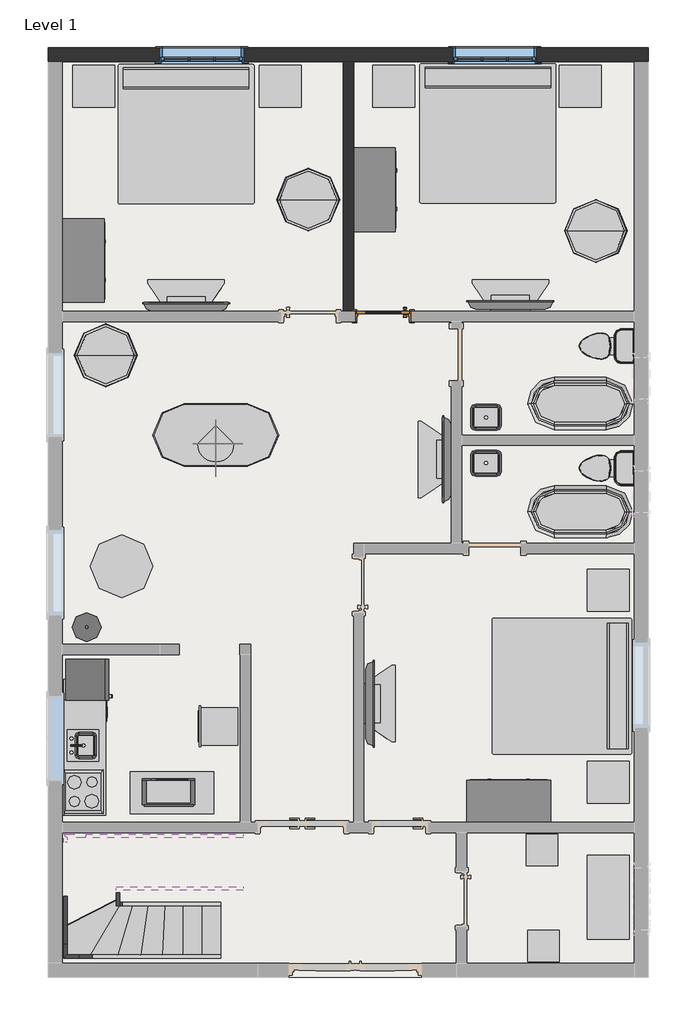
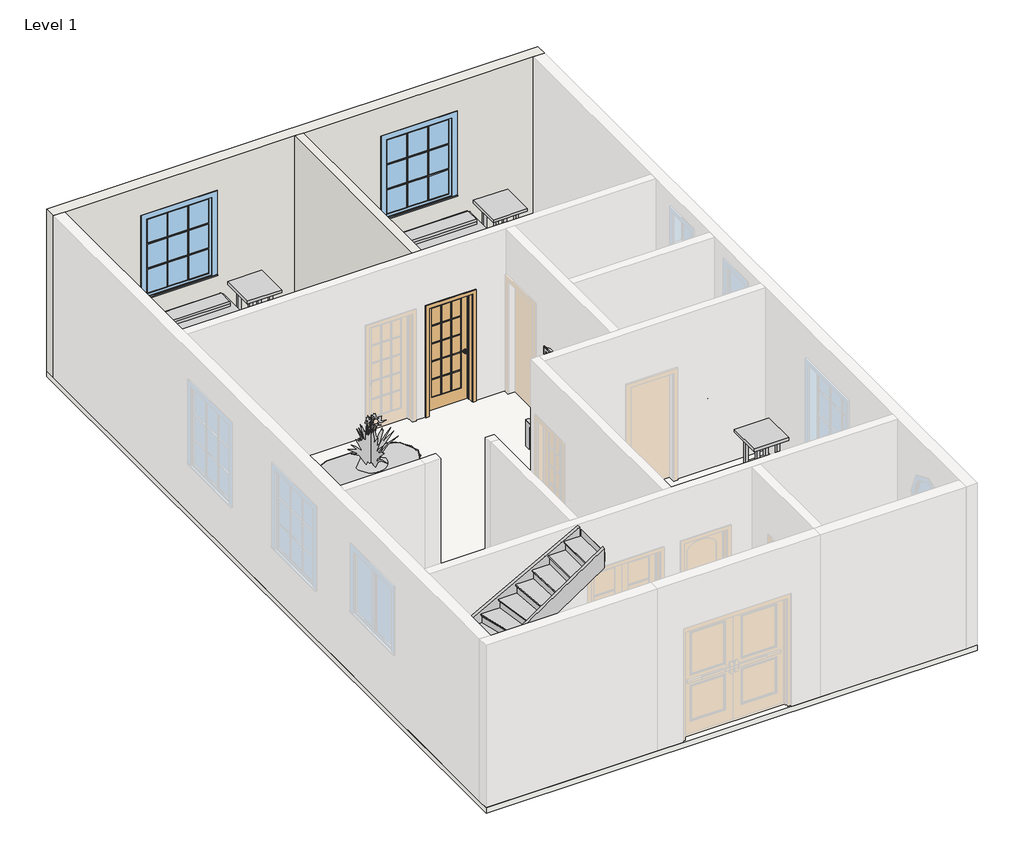
# One storey, part 2 of 2: 30 furniture elements, 10 members, 8 flow terminals, 6 proxies, 2 walls, 2 windows, 1 door, 1 geographic element, 2 other elements.
"""IFC4 building model written with IfcOpenShell, lengths in millimetres."""

from ifc_helpers import new_model, si_unit, frame, origin, origin_with_axes, place, context, project, spatial, polyline, outline, extrude, faceted_brep, transform, mapped, element, save
from components import proxy_a6faaae8, proxy_45b28599, kitchenette_medium_kitchenette_medium_844211aa, proxy_8a8d5ab2, proxy_34c9623a, proxy_c523a7b7, door_a0b5ff2a, flow_terminal_871c2e40, flow_terminal_d49f872f, flow_terminal_62a433f7, toilet_domestic_3d_toilet_domestic_3d_f7549cf7, toilet_domestic_3d_toilet_domestic_3d_183bbd19, flow_terminal_b374fae2, furniture_1fc5af50, furniture_1781b5df, furniture_9fa109b2, furniture_fdf74506, tv_stand_tv_stand_6ce107e5, furniture_2c34a4f9, furniture_905aceb5, furniture_097b63cf, furniture_5bc9ed15, furniture_51091a24, furniture_c80d6d9c, rpc_plant_tropical_55f6ff97, stair_flight_bf45dea3, window_cfa1ffdd

model = new_model("IFC4")

# Units and contexts
model_context = context("Model", 3, world=origin())
ifc_project = project(units=[si_unit("LENGTHUNIT", "METRE", prefix="MILLI")], contexts=[model_context])

# Site, building, storey
site = spatial("IfcSite", under=ifc_project)
building = spatial("IfcBuilding", under=site)
storey = spatial("IfcBuildingStorey", under=building, Name="Level 1", Elevation=0.0)

# Proxies
placement = place(None, origin())
proxy_shape = proxy_a6faaae8(model_context)
element("IfcBuildingElementProxy", 1, Name="Cook Top-4 Unit2 : 22\" x 20\"", ObjectType="Cook Top-4 Unit2 : 22\" x 20\"", at=placement, inside=storey, context=model_context, shape_type="MappedRepresentation", body=[
    mapped(proxy_shape, transform((-8710.4653968, 1396.1297533, 0.0), x_axis=(0.0, 1.0000000000000002, 0.0), y_axis=(-1.0000000000000002, 0.0, 0.0), z_axis=(0.0, 0.0, 1.0))),
])
proxy_2_shape = proxy_45b28599(model_context)
element("IfcBuildingElementProxy", 2, Name="Dishwasher : 24\" x 24\" x 34\"", ObjectType="Dishwasher : 24\" x 24\" x 34\"", at=placement, inside=storey, context=model_context, shape_type="MappedRepresentation", body=[
    mapped(proxy_2_shape, transform((-8418.6158321, 2347.3122848, 0.0), x_axis=(0.0, 1.0000000000000002, 0.0), y_axis=(-1.0000000000000002, 0.0, 0.0), z_axis=(0.0, 0.0, 1.0))),
])
kitchenette_medium_kitchenette_medium_shape = kitchenette_medium_kitchenette_medium_844211aa(model_context)
element("IfcBuildingElementProxy", 3, Name="Kitchenette - Medium : Kitchenette - Medium", ObjectType="Kitchenette - Medium : Kitchenette - Medium", at=placement, inside=storey, context=model_context, shape_type="MappedRepresentation", body=[
    mapped(kitchenette_medium_kitchenette_medium_shape, transform((-9015.2653968, 1720.2920484, 0.0), x_axis=(0.0, 1.0000000000000002, 0.0), y_axis=(-1.0000000000000002, 0.0, 0.0), z_axis=(0.0, 0.0, 1.0))),
])
proxy_3_shape = proxy_8a8d5ab2(model_context)
element("IfcBuildingElementProxy", 4, Name="Microwave : 30\" x 16\" x 18\"", ObjectType="Microwave : 30\" x 16\" x 18\"", at=placement, inside=storey, context=model_context, shape_type="MappedRepresentation", body=[
    mapped(proxy_3_shape, transform((-6965.5725195, 1030.3492475, 0.0), x_axis=(-1.0000000000000004, 0.0, 0.0), y_axis=(0.0, -1.0000000000000004, 0.0), z_axis=(0.0, 0.0, 1.0))),
])
proxy_4_shape = proxy_34c9623a(model_context)
element("IfcBuildingElementProxy", 5, Name="Oven Single-Built-in : 21\" x 23 1/2\" x 21\"", ObjectType="Oven Single-Built-in : 21\" x 23 1/2\" x 21\"", at=placement, inside=storey, context=model_context, shape_type="MappedRepresentation", body=[
    mapped(proxy_4_shape, transform((-6870.3312558, 2313.454826, 0.0), x_axis=(0.0, -1.0000000000000007, 0.0), y_axis=(1.0000000000000007, 0.0, 0.0), z_axis=(0.0, 0.0, 1.0))),
])
proxy_5_shape = proxy_c523a7b7(model_context)
element("IfcBuildingElementProxy", 6, Name="Refrigerator : 24\" x 25\" LH", ObjectType="Refrigerator : 24\" x 25\" LH", at=placement, inside=storey, context=model_context, shape_type="MappedRepresentation", body=[
    mapped(proxy_5_shape, transform((-8664.8164254, 3028.0797533, 0.0), x_axis=(0.0, 1.0000000000000002, 0.0), y_axis=(-1.0000000000000002, 0.0, 0.0), z_axis=(0.0, 0.0, 1.0))),
])

# Door
door_shape = door_a0b5ff2a(model_context)
element("IfcDoor", 7, ObjectType="Door-Interior-Single-Full Glass-Wood : 30\" x 80\"", at=placement, inside=storey, context=model_context, shape_type="MappedRepresentation", body=[
    mapped(door_shape, transform((-4341.6653968, 8320.8047533, 0.0), x_axis=(-1.0, 0.0, 0.0), y_axis=(0.0, -1.0, 0.0), z_axis=(0.0, 0.0, 1.0))),
])

# Flow terminals
flow_terminal_shape = flow_terminal_871c2e40(model_context)
element("IfcFlowTerminal", 8, ObjectType="Sink Kitchen-Island : 18\" x 18\"", at=placement, inside=storey, context=model_context, shape_type="MappedRepresentation", body=[
    mapped(flow_terminal_shape, transform((-8708.1199957, 2053.5405127, -14.4), x_axis=(0.0, 1.0000000000000002, 0.0), y_axis=(-1.0000000000000002, 0.0, 0.0), z_axis=(0.0, 0.0, 1.0))),
])
flow_terminal_2_shape = flow_terminal_d49f872f(model_context)
element("IfcFlowTerminal", 9, ObjectType="Sink Vanity-Round : 19\" x 19\"", at=placement, inside=storey, context=model_context, shape_type="MappedRepresentation", body=[
    mapped(flow_terminal_2_shape, transform((-8563.0136563, 3878.2665595, 609.6), x_axis=(-1.0000000000000004, 0.0, 0.0), y_axis=(0.0, -1.0000000000000004, 0.0), z_axis=(0.0, 0.0, 1.0))),
])
flow_terminal_3_shape = flow_terminal_62a433f7(model_context)
element("IfcFlowTerminal", 10, ObjectType="Sink Vanity-Square : 20\" x 18\"", at=placement, inside=storey, context=model_context, shape_type="MappedRepresentation", body=[
    mapped(flow_terminal_3_shape, transform((-2858.7546374, 6232.4843522, 609.6), x_axis=(1.0, 0.0, 0.0), y_axis=(0.0, 1.0, 0.0), z_axis=(0.0, 0.0, 1.0))),
])
element("IfcFlowTerminal", 11, ObjectType="Sink Vanity-Square : 20\" x 18\"", at=placement, inside=storey, context=model_context, shape_type="MappedRepresentation", body=[
    mapped(flow_terminal_3_shape, transform((-2827.3761563, 6795.9751544, 609.6), x_axis=(-1.0, 0.0, 0.0), y_axis=(0.0, -1.0, 0.0), z_axis=(0.0, 0.0, 1.0))),
])
toilet_domestic_3d_toilet_domestic_3d_shape = toilet_domestic_3d_toilet_domestic_3d_f7549cf7(model_context)
toilet_domestic_3d_toilet_domestic_3d_2_shape = toilet_domestic_3d_toilet_domestic_3d_183bbd19(model_context)
element("IfcFlowTerminal", 12, ObjectType="Toilet-Domestic-3D : Toilet-Domestic-3D", at=placement, inside=storey, context=model_context, shape_type="MappedRepresentation", body=[
    mapped(toilet_domestic_3d_toilet_domestic_3d_shape, transform((-1178.7614242, 7885.8297533, 0.0), x_axis=(0.0, -1.0000000000000002, 0.0), y_axis=(1.0000000000000002, 0.0, 0.0), z_axis=(0.0, 0.0, 1.0))),
    mapped(toilet_domestic_3d_toilet_domestic_3d_2_shape, transform((-1178.7614242, 7885.8297533, 0.0), x_axis=(0.0, -1.0000000000000002, 0.0), y_axis=(1.0000000000000002, 0.0, 0.0), z_axis=(0.0, 0.0, 1.0))),
])
element("IfcFlowTerminal", 13, ObjectType="Toilet-Domestic-3D : Toilet-Domestic-3D", at=placement, inside=storey, context=model_context, shape_type="MappedRepresentation", body=[
    mapped(toilet_domestic_3d_toilet_domestic_3d_shape, transform((-1178.7614242, 6107.8297533, 0.0), x_axis=(0.0, -1.0, 0.0), y_axis=(1.0, 0.0, 0.0), z_axis=(0.0, 0.0, 1.0))),
    mapped(toilet_domestic_3d_toilet_domestic_3d_2_shape, transform((-1178.7614242, 6107.8297533, 0.0), x_axis=(0.0, -1.0, 0.0), y_axis=(1.0, 0.0, 0.0), z_axis=(0.0, 0.0, 1.0))),
])
flow_terminal_4_shape = flow_terminal_b374fae2(model_context)
element("IfcFlowTerminal", 14, ObjectType="Tub-Free Standing-3D : 30\" x 60\"", at=placement, inside=storey, context=model_context, shape_type="MappedRepresentation", body=[
    mapped(flow_terminal_4_shape, transform((-1471.4653968, 7047.6297533, 0.0), x_axis=(0.0, -1.0000000000000002, 0.0), y_axis=(1.0000000000000002, 0.0, 0.0), z_axis=(0.0, 0.0, 1.0))),
])
element("IfcFlowTerminal", 15, ObjectType="Tub-Free Standing-3D : 30\" x 60\"", at=placement, inside=storey, context=model_context, shape_type="MappedRepresentation", body=[
    mapped(flow_terminal_4_shape, transform((-1471.4653968, 5472.8297533, 0.0), x_axis=(0.0, -1.0, 0.0), y_axis=(1.0, 0.0, 0.0), z_axis=(0.0, 0.0, 1.0))),
])

# Furniture
furniture_shape = furniture_1fc5af50(model_context)
element("IfcFurniture", 16, ObjectType="Bed-Standard.0001 : King 78\" x 80\"", at=placement, inside=storey, context=model_context, shape_type="MappedRepresentation", body=[
    mapped(furniture_shape, transform((-7483.3539214, 11017.5248353, 0.0), x_axis=(1.0, 0.0, 0.0), y_axis=(0.0, 1.0, 0.0), z_axis=(0.0, 0.0, 1.0))),
])
element("IfcFurniture", 17, ObjectType="Bed-Standard.0001 : King 78\" x 80\"", at=placement, inside=storey, context=model_context, shape_type="MappedRepresentation", body=[
    mapped(furniture_shape, transform((-3089.1539214, 11030.2248353, 0.0), x_axis=(1.0, 0.0, 0.0), y_axis=(0.0, 1.0, 0.0), z_axis=(0.0, 0.0, 1.0))),
])
element("IfcFurniture", 18, ObjectType="Bed-Standard.0001 : King 78\" x 80\"", at=placement, inside=storey, context=model_context, shape_type="MappedRepresentation", body=[
    mapped(furniture_shape, transform((-1692.5703149, 3204.3182779, 0.0), x_axis=(0.0, -1.0000000000000004, 0.0), y_axis=(1.0000000000000004, 0.0, 0.0), z_axis=(0.0, 0.0, 1.0))),
])
furniture_2_shape = furniture_1781b5df(model_context)
element("IfcFurniture", 19, ObjectType="Counter Top w Sink Hole : 24\" Depth", at=placement, inside=storey, context=model_context, shape_type="MappedRepresentation", body=[
    mapped(furniture_2_shape, transform((-9015.2653968, 2253.6920484, -14.4), x_axis=(0.0, 1.0000000000000002, 0.0), y_axis=(-1.0000000000000002, 0.0, 0.0), z_axis=(0.0, 0.0, 1.0))),
])
furniture_3_shape = furniture_9fa109b2(model_context)
element("IfcFurniture", 20, ObjectType="Dresser : 48\" x 72\" x 24\"", at=placement, inside=storey, context=model_context, shape_type="MappedRepresentation", body=[
    mapped(furniture_3_shape, transform((-9073.6283509, 9399.6230131, 0.0), x_axis=(0.0, 1.0000000000000002, 0.0), y_axis=(-1.0000000000000002, 0.0, 0.0), z_axis=(0.0, 0.0, 1.0))),
])
element("IfcFurniture", 21, ObjectType="Dresser : 48\" x 72\" x 24\"", at=placement, inside=storey, context=model_context, shape_type="MappedRepresentation", body=[
    mapped(furniture_3_shape, transform((-4831.8283509, 10430.8404811, 0.0), x_axis=(0.0, 1.0000000000000002, 0.0), y_axis=(-1.0000000000000002, 0.0, 0.0), z_axis=(0.0, 0.0, 1.0))),
])
element("IfcFurniture", 22, ObjectType="Dresser : 48\" x 72\" x 24\"", at=placement, inside=storey, context=model_context, shape_type="MappedRepresentation", body=[
    mapped(furniture_3_shape, transform((-2782.0586567, 893.2667992, 0.0), x_axis=(-1.0000000000000002, 0.0, 0.0), y_axis=(0.0, -1.0000000000000002, 0.0), z_axis=(0.0, 0.0, 1.0))),
])
furniture_4_shape = furniture_fdf74506(model_context)
element("IfcFurniture", 23, ObjectType="TV - Flat Screen : 50\"", at=placement, inside=storey, context=model_context, shape_type="MappedRepresentation", body=[
    mapped(furniture_4_shape, transform((-7215.809911, 8452.3683769, 914.4), x_axis=(-1.0, 0.0, 0.0), y_axis=(0.0, -1.0, 0.0), z_axis=(0.0, 0.0, 1.0))),
])
element("IfcFurniture", 24, ObjectType="TV - Flat Screen : 50\"", at=placement, inside=storey, context=model_context, shape_type="MappedRepresentation", body=[
    mapped(furniture_4_shape, transform((-2491.409911, 8477.7683769, 914.4), x_axis=(-1.0, 0.0, 0.0), y_axis=(0.0, -1.0, 0.0), z_axis=(0.0, 0.0, 1.0))),
])
element("IfcFurniture", 25, ObjectType="TV - Flat Screen : 50\"", at=placement, inside=storey, context=model_context, shape_type="MappedRepresentation", body=[
    mapped(furniture_4_shape, transform((-4537.1267732, 2682.7742674, 914.4), x_axis=(0.0, 1.0000000000000002, 0.0), y_axis=(-1.0000000000000002, 0.0, 0.0), z_axis=(0.0, 0.0, 1.0))),
])
element("IfcFurniture", 26, ObjectType="TV - Flat Screen : 50\"", at=placement, inside=storey, context=model_context, shape_type="MappedRepresentation", body=[
    mapped(furniture_4_shape, transform((-3409.6040205, 6230.8852392, 914.4), x_axis=(0.0, -1.0000000000000002, 0.0), y_axis=(1.0000000000000002, 0.0, 0.0), z_axis=(0.0, 0.0, 1.0))),
])
tv_stand_tv_stand_shape = tv_stand_tv_stand_6ce107e5(model_context)
element("IfcFurniture", 27, ObjectType="TV Stand : TV Stand", at=placement, inside=storey, context=model_context, shape_type="MappedRepresentation", body=[
    mapped(tv_stand_tv_stand_shape, transform((-7086.6773948, 8393.8297533, 0.0), x_axis=(-1.0000000000000004, 0.0, 0.0), y_axis=(0.0, -1.0000000000000004, 0.0), z_axis=(0.0, 0.0, 1.0))),
])
element("IfcFurniture", 28, ObjectType="TV Stand : TV Stand", at=placement, inside=storey, context=model_context, shape_type="MappedRepresentation", body=[
    mapped(tv_stand_tv_stand_shape, transform((-2362.2773948, 8393.8297533, 0.0), x_axis=(-1.0, 0.0, 0.0), y_axis=(0.0, -1.0, 0.0), z_axis=(0.0, 0.0, 1.0))),
])
element("IfcFurniture", 29, ObjectType="TV Stand : TV Stand", at=placement, inside=storey, context=model_context, shape_type="MappedRepresentation", body=[
    mapped(tv_stand_tv_stand_shape, transform((-4621.0653968, 2553.6417512, 0.0), x_axis=(0.0, 1.0000000000000004, 0.0), y_axis=(-1.0000000000000004, 0.0, 0.0), z_axis=(0.0, 0.0, 1.0))),
])
element("IfcFurniture", 30, ObjectType="TV Stand : TV Stand", at=placement, inside=storey, context=model_context, shape_type="MappedRepresentation", body=[
    mapped(tv_stand_tv_stand_shape, transform((-3376.4653968, 6360.0177554, 0.0), x_axis=(0.0, -1.0, 0.0), y_axis=(1.0, 0.0, 0.0), z_axis=(0.0, 0.0, 1.0))),
])
furniture_5_shape = furniture_2c34a4f9(model_context)
element("IfcFurniture", 31, ObjectType="Table-Dining Oval : 36\" x 72\"", at=placement, inside=storey, context=model_context, shape_type="MappedRepresentation", body=[
    mapped(furniture_5_shape, transform((-6378.2457247, 6948.528114, 0.0), x_axis=(1.0, 0.0, 0.0), y_axis=(0.0, 1.0, 0.0), z_axis=(0.0, 0.0, 1.0))),
])
furniture_6_shape = furniture_905aceb5(model_context)
element("IfcFurniture", 32, ObjectType="Table-Dining Round w Chairs : 36\" Diameter", at=placement, inside=storey, context=model_context, shape_type="MappedRepresentation", body=[
    mapped(furniture_6_shape, transform((-8255.3473641, 4863.9584418, 0.0), x_axis=(1.0, 0.0, 0.0), y_axis=(0.0, 1.0, 0.0), z_axis=(0.0, 0.0, 1.0))),
])
furniture_7_shape = furniture_097b63cf(model_context)
element("IfcFurniture", 33, ObjectType="Table-Night Stand : 18\" x 18\" x 24\"", at=placement, inside=storey, context=model_context, shape_type="MappedRepresentation", body=[
    mapped(furniture_7_shape, transform((-2262.5990271, 316.6297533, 0.0), x_axis=(1.0, 0.0, 0.0), y_axis=(0.0, 1.0, 0.0), z_axis=(0.0, 0.0, 1.0))),
])
element("IfcFurniture", 34, ObjectType="Table-Night Stand : 18\" x 18\" x 24\"", at=placement, inside=storey, context=model_context, shape_type="MappedRepresentation", body=[
    mapped(furniture_7_shape, transform((-2237.1990271, -1080.3702467, 0.0), x_axis=(1.0, 0.0, 0.0), y_axis=(0.0, 1.0, 0.0), z_axis=(0.0, 0.0, 1.0))),
])
furniture_8_shape = furniture_5bc9ed15(model_context)
element("IfcFurniture", 35, ObjectType="Table-Night Stand : 24\" x 24\" x 30\"", at=placement, inside=storey, context=model_context, shape_type="MappedRepresentation", body=[
    mapped(furniture_8_shape, transform((-1373.5990271, 4025.0297533, 0.0), x_axis=(1.0, 0.0, 0.0), y_axis=(0.0, 1.0, 0.0), z_axis=(0.0, 0.0, 1.0))),
])
element("IfcFurniture", 36, ObjectType="Table-Night Stand : 24\" x 24\" x 30\"", at=placement, inside=storey, context=model_context, shape_type="MappedRepresentation", body=[
    mapped(furniture_8_shape, transform((-1373.5990271, 1231.0297533, 0.0), x_axis=(1.0, 0.0, 0.0), y_axis=(0.0, 1.0, 0.0), z_axis=(0.0, 0.0, 1.0))),
])
element("IfcFurniture", 37, ObjectType="Table-Night Stand : 24\" x 24\" x 30\"", at=placement, inside=storey, context=model_context, shape_type="MappedRepresentation", body=[
    mapped(furniture_8_shape, transform((-8866.5990271, 11365.6297533, 0.0), x_axis=(1.0, 0.0, 0.0), y_axis=(0.0, 1.0, 0.0), z_axis=(0.0, 0.0, 1.0))),
])
element("IfcFurniture", 38, ObjectType="Table-Night Stand : 24\" x 24\" x 30\"", at=placement, inside=storey, context=model_context, shape_type="MappedRepresentation", body=[
    mapped(furniture_8_shape, transform((-6148.7990271, 11365.6297533, 0.0), x_axis=(1.0, 0.0, 0.0), y_axis=(0.0, 1.0, 0.0), z_axis=(0.0, 0.0, 1.0))),
])
element("IfcFurniture", 39, ObjectType="Table-Night Stand : 24\" x 24\" x 30\"", at=placement, inside=storey, context=model_context, shape_type="MappedRepresentation", body=[
    mapped(furniture_8_shape, transform((-4497.7990271, 11365.6297533, 0.0), x_axis=(1.0, 0.0, 0.0), y_axis=(0.0, 1.0, 0.0), z_axis=(0.0, 0.0, 1.0))),
])
element("IfcFurniture", 40, ObjectType="Table-Night Stand : 24\" x 24\" x 30\"", at=placement, inside=storey, context=model_context, shape_type="MappedRepresentation", body=[
    mapped(furniture_8_shape, transform((-1779.9990271, 11365.6297533, 0.0), x_axis=(1.0, 0.0, 0.0), y_axis=(0.0, 1.0, 0.0), z_axis=(0.0, 0.0, 1.0))),
])
furniture_9_shape = furniture_51091a24(model_context)
element("IfcFurniture", 41, ObjectType="Table-Rectangular : 72\" x 30\"", at=placement, inside=storey, context=model_context, shape_type="MappedRepresentation", body=[
    mapped(furniture_9_shape, transform((-1065.0653968, -140.5702467, 0.0), x_axis=(0.0, 1.0000000000000002, 0.0), y_axis=(-1.0000000000000002, 0.0, 0.0), z_axis=(0.0, 0.0, 1.0))),
])
element("IfcFurniture", 42, ObjectType="Table-Rectangular : 72\" x 30\"", at=placement, inside=storey, context=model_context, shape_type="MappedRepresentation", body=[
    mapped(furniture_9_shape, transform((-7415.0653968, 1383.4297533, 0.0), x_axis=(1.0, 0.0, 0.0), y_axis=(0.0, 1.0, 0.0), z_axis=(0.0, 0.0, 1.0))),
])
furniture_10_shape = furniture_c80d6d9c(model_context)
element("IfcFurniture", 43, ObjectType="Table-Round : 36\" Diameter", at=placement, inside=storey, context=model_context, shape_type="MappedRepresentation", body=[
    mapped(furniture_10_shape, transform((-5433.8653968, 10019.4297533, 0.0), x_axis=(1.0, 0.0, 0.0), y_axis=(0.0, 1.0, 0.0), z_axis=(0.0, 0.0, 1.0))),
])
element("IfcFurniture", 44, ObjectType="Table-Round : 36\" Diameter", at=placement, inside=storey, context=model_context, shape_type="MappedRepresentation", body=[
    mapped(furniture_10_shape, transform((-1242.8653968, 9562.2297533, 0.0), x_axis=(1.0, 0.0, 0.0), y_axis=(0.0, 1.0, 0.0), z_axis=(0.0, 0.0, 1.0))),
])
element("IfcFurniture", 45, ObjectType="Table-Round : 36\" Diameter", at=placement, inside=storey, context=model_context, shape_type="MappedRepresentation", body=[
    mapped(furniture_10_shape, transform((-8380.2653968, 7752.4797533, 0.0), x_axis=(1.0, 0.0, 0.0), y_axis=(0.0, 1.0, 0.0), z_axis=(0.0, 0.0, 1.0))),
])

# Geographic element
rpc_plant_tropical_shape = rpc_plant_tropical_55f6ff97(model_context)
element("IfcGeographicElement", 46, ObjectType="RPC Plant - Tropical", at=placement, inside=storey, context=model_context, shape_type="MappedRepresentation", body=[
    mapped(rpc_plant_tropical_shape, transform((-6780.0653968, 6463.4297533, 914.4), x_axis=(1.0, 0.0, 0.0), y_axis=(0.0, 1.0, 0.0), z_axis=(0.0, 0.0, 1.0))),
])

# Members
element("IfcMember", 47, ObjectType="Stringer - 2\" Width", at=placement, inside=storey, context=model_context, shape_type="SweptSolid", body=[
    extrude(outline(polyline([(0.0, -6703.8653968), (228.5330317, -6703.8653968), (1305.4011192, -8771.2543536), (961.730602, -8771.2543536), (0.0, -6924.9082236), (0.0, -6703.8653968)])), frame((0.0, -1029.5702467, 0.0), z_axis=(0.0, 1.0, 0.0), x_axis=(0.0, 0.0, 1.0)), (0.0, 0.0, 1.0), 50.8),
])
element("IfcMember", 48, ObjectType="Stringer - 2\" Width", at=placement, inside=storey, context=model_context, shape_type="SweptSolid", body=[
    extrude(outline(polyline([(-8771.2543536, -978.7702467), (-8771.2543536, -1029.5702467), (-8993.5970887, -1029.5702467), (-8942.7970887, -978.7702467), (-8771.2543536, -978.7702467)])), frame((0.0, 0.0, 961.730602), z_axis=(0.0, 0.0, 1.0), x_axis=(1.0, 0.0, 0.0)), (0.0, 0.0, 1.0), 343.6705172),
])
element("IfcMember", 49, ObjectType="Stringer - 2\" Width", at=placement, inside=storey, context=model_context, shape_type="SweptSolid", body=[
    extrude(outline(polyline([(-8942.7970887, -978.7702467), (-8993.5970887, -1029.5702467), (-8993.5970887, -827.9218653), (-8942.7970887, -827.9218653), (-8942.7970887, -978.7702467)])), frame((0.0, 0.0, 961.730602), z_axis=(0.0, 0.0, 1.0), x_axis=(1.0, 0.0, 0.0)), (0.0, 0.0, 1.0), 343.6705172),
])
element("IfcMember", 50, ObjectType="Stringer - 2\" Width", at=placement, inside=storey, context=model_context, shape_type="SweptSolid", body=[
    extrude(outline(polyline([(-827.9218653, 961.730602), (-827.9218653, 1305.4011192), (662.2844822, 1813.4011192), (662.2844822, 1469.730602), (-827.9218653, 961.730602)])), frame((-8993.5970887, 0.0, 0.0), z_axis=(1.0, 0.0, 0.0), x_axis=(0.0, 1.0, 0.0)), (0.0, 0.0, 1.0), 50.8),
])
element("IfcMember", 51, ObjectType="Stringer - 2\" Width", at=placement, inside=storey, context=model_context, shape_type="SweptSolid", body=[
    extrude(outline(polyline([(-8942.7970887, 662.2844822), (-8993.5970887, 662.2844822), (-8993.5970887, 773.8297533), (-8942.7970887, 723.0297533), (-8942.7970887, 662.2844822)])), frame((0.0, 0.0, 1479.9551215), z_axis=(0.0, 0.0, 1.0), x_axis=(1.0, 0.0, 0.0)), (0.0, 0.0, 1.0), 322.0234171),
])
element("IfcMember", 52, ObjectType="Stringer - 2\" Width", at=placement, inside=storey, context=model_context, shape_type="SweptSolid", body=[
    extrude(outline(polyline([(0.0, -6703.8653968), (194.5849337, -6703.8653968), (1234.3238531, -8180.7970887), (861.5700283, -8180.7970887), (0.0, -6956.9513176), (0.0, -6703.8653968)])), frame((0.0, -267.5702467, 0.0), z_axis=(0.0, 1.0, 0.0), x_axis=(0.0, 0.0, 1.0)), (0.0, 0.0, 1.0), 50.8),
])
element("IfcMember", 53, ObjectType="Stringer - 2\" Width", at=placement, inside=storey, context=model_context, shape_type="SweptSolid", body=[
    extrude(outline(polyline([(-267.5702467, 897.3325063), (-267.5702467, 1478.2726464), (-53.2751767, 1871.3232191), (-38.9702467, 1871.3232191), (-38.9702467, 1260.8183928), (-237.1463566, 897.3325063), (-267.5702467, 897.3325063)])), frame((-8231.5970887, 0.0, 0.0), z_axis=(1.0, 0.0, 0.0), x_axis=(0.0, 1.0, 0.0)), (0.0, 0.0, 1.0), 50.8),
])
element("IfcMember", 54, ObjectType="Stringer - 2\" Width", at=placement, inside=storey, context=model_context, shape_type="SweptSolid", body=[
    extrude(outline(polyline([(1871.3232191, -8231.5970887), (1503.9377762, -8231.5970887), (2748.6444185, -6381.8994015), (3116.0298613, -6381.8994015), (1871.3232191, -8231.5970887)])), frame((0.0, -38.9702467, 0.0), z_axis=(0.0, 1.0, 0.0), x_axis=(0.0, 0.0, 1.0)), (0.0, 0.0, 1.0), 50.8),
])
element("IfcMember", 55, ObjectType="Stringer - 2\" Width", at=placement, inside=storey, context=model_context, shape_type="SweptSolid", body=[
    extrude(outline(polyline([(-8942.7970887, 723.0297533), (-8993.5970887, 773.8297533), (-8673.8690979, 773.8297533), (-8673.8690979, 723.0297533), (-8942.7970887, 723.0297533)])), frame((0.0, 0.0, 1479.9551215), z_axis=(0.0, 0.0, 1.0), x_axis=(1.0, 0.0, 0.0)), (0.0, 0.0, 1.0), 322.0234171),
])
element("IfcMember", 56, ObjectType="Stringer - 2\" Width", at=placement, inside=storey, context=model_context, shape_type="SweptSolid", body=[
    extrude(outline(polyline([(1801.9785386, -8673.8690979), (1479.9551215, -8673.8690979), (2733.4245791, -6381.8994015), (3055.4479962, -6381.8994015), (1801.9785386, -8673.8690979)])), frame((0.0, 723.0297533, 0.0), z_axis=(0.0, 1.0, 0.0), x_axis=(0.0, 0.0, 1.0)), (0.0, 0.0, 1.0), 50.8),
])

# Slab
element("IfcSlab", 57, ObjectType="LW Concrete on Metal Deck", at=placement, inside=storey, context=model_context, shape_type="SweptSolid", body=[
    extrude(outline(polyline([(-480.8653968, 12229.2297533), (-480.8653968, -1308.9702467), (-9218.4653968, -1308.9702467), (-9218.4653968, 12229.2297533), (-480.8653968, 12229.2297533)])), frame((0.0, 0.0, -104.775), z_axis=(0.0, 0.0, 1.0), x_axis=(1.0, 0.0, 0.0)), (0.0, 0.0, 1.0), 104.775),
])

# Stair flight
stair_flight_shape = stair_flight_bf45dea3(model_context)
element("IfcStairFlight", 58, ObjectType="2\" Tread 1\" Nosing 1/4\" Riser", at=placement, inside=storey, context=model_context, shape_type="MappedRepresentation", body=[
    mapped(stair_flight_shape, transform((0.0, 0.0, 0.0), x_axis=(1.0, 0.0, 0.0), y_axis=(0.0, 1.0, 0.0), z_axis=(0.0, 0.0, 1.0))),
])

# Walls
element("IfcWall", 59, ObjectType="Generic - 8\"", at=placement, inside=storey, context=model_context, shape_type="Brep", body=[
    faceted_brep([(-9218.4653968, 12026.0297533, 0.0), (-9015.2653968, 12026.0297533, 0.0), (-4925.8653968, 12026.0297533, 0.0), (-4773.4653968, 12026.0297533, 0.0), (-684.0653968, 12026.0297533, 0.0), (-480.8653968, 12026.0297533, 0.0), (-480.8653968, 12026.0297533, 3048.0), (-684.0653968, 12026.0297533, 3048.0), (-4773.4653968, 12026.0297533, 3048.0), (-4925.8653968, 12026.0297533, 3048.0), (-9015.2653968, 12026.0297533, 3048.0), (-9218.4653968, 12026.0297533, 3048.0), (-7592.8653968, 12026.0297533, 2438.4), (-6373.6653968, 12026.0297533, 2438.4), (-6373.6653968, 12026.0297533, 914.4), (-7592.8653968, 12026.0297533, 914.4), (-3325.6653968, 12026.0297533, 2438.4), (-2106.4653968, 12026.0297533, 2438.4), (-2106.4653968, 12026.0297533, 914.4), (-3325.6653968, 12026.0297533, 914.4), (-9218.4653968, 12229.2297533, 0.0), (-9218.4653968, 12229.2297533, 3048.0), (-480.8653968, 12229.2297533, 3048.0), (-480.8653968, 12229.2297533, 0.0), (-7592.8653968, 12229.2297533, 2438.4), (-7592.8653968, 12229.2297533, 914.4), (-6373.6653968, 12229.2297533, 914.4), (-6373.6653968, 12229.2297533, 2438.4), (-3325.6653968, 12229.2297533, 2438.4), (-3325.6653968, 12229.2297533, 914.4), (-2106.4653968, 12229.2297533, 914.4), (-2106.4653968, 12229.2297533, 2438.4)], [[[0, 1, 2, 3, 4, 5, 6, 7, 8, 9, 10, 11], [12, 13, 14, 15], [16, 17, 18, 19]], [[20, 21, 22, 23], [24, 25, 26, 27], [28, 29, 30, 31]], [[5, 4, 3, 2, 1, 0, 20, 23]], [[6, 5, 23, 22]], [[0, 11, 21, 20]], [[25, 24, 12, 15]], [[26, 25, 15, 14]], [[27, 26, 14, 13]], [[24, 27, 13, 12]], [[29, 28, 16, 19]], [[30, 29, 19, 18]], [[31, 30, 18, 17]], [[28, 31, 17, 16]], [[11, 10, 9, 8, 7, 6, 22, 21]]]),
])
element("IfcWall", 60, ObjectType="INNER WALL", at=placement, inside=storey, context=model_context, shape_type="SweptSolid", body=[
    extrude(outline(polyline([(-4925.8653968, 8393.8297533), (-4925.8653968, 12026.0297533), (-4773.4653968, 12026.0297533), (-4773.4653968, 8393.8297533), (-4925.8653968, 8393.8297533)])), origin_with_axes(), (0.0, 0.0, 1.0), 3048.0),
])

# Windows
window_shape = window_cfa1ffdd(model_context)
element("IfcWindow", 61, ObjectType="Casement 3x3 with Trim : 48\" x 60\"", at=placement, inside=storey, context=model_context, shape_type="MappedRepresentation", body=[
    mapped(window_shape, transform((-6983.2653968, 12127.6297533, 304.8), x_axis=(-1.0, 0.0, 0.0), y_axis=(0.0, -1.0, 0.0), z_axis=(0.0, 0.0, 1.0))),
])
element("IfcWindow", 62, ObjectType="Casement 3x3 with Trim : 48\" x 60\"", at=placement, inside=storey, context=model_context, shape_type="MappedRepresentation", body=[
    mapped(window_shape, transform((-2716.0653968, 12127.6297533, 304.8), x_axis=(-1.0, 0.0, 0.0), y_axis=(0.0, -1.0, 0.0), z_axis=(0.0, 0.0, 1.0))),
])

save(model, "model.ifc")

# Revit data of these elements
# Type "Cook Top-4 Unit2 : 22\" x 20\""
#   Depth = 1' - 8"
#   Width = 1' - 10"
#   Burner Material = Steel, Chrome Plated
#   Cooktop Material = Steel, Polished
#   Default Elevation = 0
#   Assembly Code = ""
# Type "Dishwasher : 24\" x 24\" x 34\""
#   Label = "DW"
#   Assembly Code = "E1090400"
#   Depth = 2' - 0"
#   Height = 2' - 10"
#   Width = 2' - 0"
#   Dishwasher Material = Steel, Paint Finish, Ivory, Glossy
#   Panel Face Material = Plastic, Opaque Black
#   Default Elevation = 0
# Type "Kitchenette - Medium : Kitchenette - Medium"
#   Assembly Code = "E1090400"
#   Counter Length = 5' - 6"
#   Cabinet Width = 4' - 6"
#   Cabinet Height = 2' - 10 1/2"
#   Cabinet Depth = 2' - 0"
#   Toe Depth = 0' - 3"
#   Toe Height = 0' - 3 1/2"
#   Cabinet Material = Cabinets
#   Door/Drawer Material = Cabinets
#   Handle Material = Cabinets - Handles
#   Default Elevation = 0
# Type "Microwave : 30\" x 16\" x 18\""
#   Assembly Code = "E1090400"
#   Depth = 1' - 4"
#   Height = 1' - 6"
#   Width = 2' - 6"
#   Microwave Material = Laminate, Ivory, Matte
#   Default Elevation = 0
# Type "Oven Single-Built-in : 21\" x 23 1/2\" x 21\""
#   Label = "OVEN"
#   Assembly Code = "E1090400"
#   Depth = 1' - 9"
#   Height = 1' - 11 1/2"
#   Install Height = 0' - 9 1/2"
#   Width = 1' - 9 1/2"
#   Oven Material = Metal - Stainless Steel, Polished
#   Default Elevation = 0
# Type "Refrigerator : 24\" x 25\" LH"
#   Label = "REF."
#   Assembly Code = "E1090400"
#   Depth = 2' - 0 3/4"
#   Handle = 0' - 1 1/2"
#   Height = 5' - 3 1/2"
#   Rear Clearance = 0' - 2"
#   Top Door Height = 1' - 8"
#   Width = 1' - 11 1/2"
#   Material = Steel, Paint Finish, Ivory, Glossy
#   Default Elevation = 0
# Type "Door-Interior-Single-Full Glass-Wood : 30\" x 80\""
#   Type Mark = "11"
#   Assembly Code = "C1020300"
#   Analytic Construction = "Wood frame with single clear glass"
#   Top Rail = 0' - 4 11/16"
#   Thickness = 0' - 1 3/8"
#   Thermal Resistance (R) = 1.0102 (h·ft²·°F)/BTU
#   Swing Angle [instance default] = 90.00°
#   Stiles = 0' - 4 3/4"
#   Rough Width = 2' - 8"
#   Rough Height = 6' - 9"
#   Height = 6' - 8"
#   Width = 2' - 6"
#   Heat Transfer Coefficient (U) = 0.9900 BTU/(h·ft²·°F)
#   Bottom Rail = 0' - 9 1/8"
#   Show Grill [instance default] = yes
#   Trim Material = Cherry
#   Panel Material = Cherry
#   Frame Material = Cherry
#   Door Handle Material = Aluminum
#   Visual Light Transmittance = 0
#   Solar Heat Gain Coefficient = 0
#   Wall Closure = (empty or 0)
#   Function = (empty or 0)
# Type "Sink Kitchen-Island : 18\" x 18\""
#   Assembly Code = "D2010410"
#   Counter Height = 3' - 0"
#   Depth = 1' - 6"
#   Width = 1' - 6"
#   Faucet Material = Steel, Polished
#   Sink Material = Steel, Polished
#   Default Elevation = 0
# Type "Sink Vanity-Round : 19\" x 19\""
#   Assembly Code = "D2010400"
#   Top Of Counter = 2' - 7"
#   Basin Material = Porcelain, Linen
#   Faucet Material = Steel, Polished
#   Default Elevation = 0
# Type "Sink Vanity-Square : 20\" x 18\""
#   Assembly Code = "D2010400"
#   Counter Height = 2' - 7"
#   Depth = 1' - 6"
#   Width = 1' - 8"
#   Basin Material = Porcelain, Linen
#   Faucet Material = Steel, Polished
#   Default Elevation = 0
# Type "Toilet-Domestic-3D : Toilet-Domestic-3D"
#   Assembly Code = "D2010110"
#   Toilet - Bowl/Basin Material = Porcelain, Linen
#   Toilet - Seat Material = Laminate, Linen, Matte
#   Default Elevation = 0
# Type "Tub-Free Standing-3D : 30\" x 60\""
#   Assembly Code = "D2010110"
#   Height = 1' - 6"
#   Length = 5' - 0"
#   Width = 2' - 6"
#   Tub Material = Porcelain, Ivory
#   Default Elevation = 0
# Type "Bed-Standard.0001 : King 78\" x 80\""
#   Assembly Code = "E2020200"
#   Length = 6' - 8"
#   Width = 6' - 6"
#   Leg Material = Steel, Chrome Plated
#   Mattress Material = Linen, White
#   Default Elevation = 0
# Type "Counter Top w Sink Hole : 24\" Depth"
#   Assembly Code = "C1030400"
#   Counter Thickness = 0' - 1 1/2"
#   Depth = 2' - 1"
#   Height = 3' - 0"
#   Length [instance default] = 8' - 0"
#   Sink Location [instance default] = 2' - 0"
#   Sink Location To Wall [instance default] = 0' - 6"
#   Sink Opening Depth [instance default] = 1' - 3"
#   Sink Opening Width [instance default] = 2' - 3"
#   Counter Top Material = none
#   Default Elevation = 0
# Type "Dresser : 48\" x 72\" x 24\""
#   Assembly Code = "E2020200"
#   Depth = 2' - 0"
#   Height = 6' - 0"
#   Width = 4' - 0"
#   Dresser Material = Laminate - Ivory, Glossy
#   Drawer Material = Laminate, Ivory, Matte
#   Knob Material = Cherry
#   Default Elevation = 0
# Type "TV - Flat Screen : 50\""
#   SinAng = 0' - 0.0193"
#   L = 3' - 7.57782"
#   H = 2' - 0.51477"
#   Thickness = 0' - 4.33071"
#   Diagonal = 4' - 2"
#   CosAng = 0' - 0.03431"
#   Stand [instance default] = yes
#   Default Elevation = 0
# Type "TV Stand : TV Stand"
#   Depth = 1' - 6"
#   Width = 3' - 8"
#   Height = 1' - 7 1/2"
#   Finish = Melamine - Gray
#   Default Elevation = 0
# Type "Table-Dining Oval : 36\" x 72\""
#   Assembly Code = "E2020200"
#   Length = 6' - 0"
#   Width = 3' - 0"
#   Base Material = Steel, Chrome Plated
#   Top Material = Glass - Clear, Grey
#   Default Elevation = 0
#   Description = (empty or 0)
# Type "Table-Dining Round w Chairs : 36\" Diameter"
#   Assembly Code = "E2020200"
#   Radius = 1' - 6"
#   Diameter = 3' - 0"
#   Height = 2' - 6"
#   Chairs = 4
#   Base Material = Pine
#   Top Material = Laminate, Linen, Matte
#   Default Elevation = 0
# Type "Table-Night Stand : 18\" x 18\" x 24\""
#   Assembly Code = "E2020200"
#   Depth = 1' - 6"
#   Height = 2' - 0"
#   Width = 1' - 6"
#   Base Material = Birch
#   Top Material = Laminate, Ivory, Matte
#   Default Elevation = 0
# Type "Table-Night Stand : 24\" x 24\" x 30\""
#   Assembly Code = "E2020200"
#   Depth = 2' - 0"
#   Height = 2' - 6"
#   Width = 2' - 0"
#   Base Material = Birch
#   Top Material = Laminate, Ivory, Matte
#   Default Elevation = 0
# Type "Table-Rectangular : 72\" x 30\""
#   Assembly Code = "E2020200"
#   Height = 2' - 6"
#   Length = 4' - 0"
#   Width = 2' - 0"
#   Base Material = Birch
#   Top Material = Birch
#   Default Elevation = 0
# Type "Table-Round : 36\" Diameter"
#   Assembly Code = "E2020200"
#   Base Radius = 0' - 10"
#   Height = 2' - 6"
#   Radius = 1' - 6"
#   Base Material = Steel, Chrome Plated
#   Top Material = Birch
#   Default Elevation = 0
# Type "RPC Plant - Tropical"
#   built-in parameter 1005198 = "{2, 15},{39, RPC-16-FWM5-GM7X-C67P-4000-ST1L-LVER-AU},{1, 0},{1, 0},{2, 13},{1, 8},{5, Color},{1, 0},{1, 0},{3, 0.8},{3, 0.8},{3, 0.8},{1, 8},{7, BBoxMin},{1, 0},{1, 0},{1, 0},{1, 0},{1, 0},{1, 8},{7, BBoxMax},{1, 0},{1, 0},{1, 0},{1, 0},{1, 0},{2, 11},{9, RPCTypeId},{1, 0},{1, 0},{39, RPC-16-FWM5-GM7X-C67P-4000-ST1L-LVER-AU},{1, 6},{14, RPCPlantHeight},{1, 0},{1, 0},{1, 3},{2, 11},{7, keyword},{1, 0},{1, 0},{35, :RPCs:Shrubs [General]:Geometry:RPC},{2, 11},{8, category},{1, 0},{1, 0},{16, Shrubs [General]},{2, 11},{12, LocalizedUID},{1, 0},{1, 0},{10, Crane Lily},{2, 14},{6, Height},{1, 0},{1, 0},{1, 3},{1, 2},{16, Cast Reflections},{1, 0},{1, 0},{1, 0},{1, 2},{12, Cast Shadows},{1, 0},{1, 0},{1, 1},{1, 2},{9, Lock View},{1, 0},{1, 0},{1, 0},{1, 4},{5, ViewC},{1, 0},{1, 0},{1, 0},{21, assetlibrary_base.fbx},{1, 5},"
#   built-in parameter 1005195 = "RPC-16-FWM5-GM7X-C67P-4000-ST1L-LVER-AU"
#   Assembly Code = "G2050500"
#   Height = 3' - 0"
#   Default Elevation = 0
# Type "LW Concrete on Metal Deck"
#   Assembly Code = "B1010"
#   Function = 0
#   Layers, outside or top first: 0' - 4" "Concrete, Lightweight" (function 1); 0' - 0 1/8" "Metal Deck" (function 1)
# Type "Generic - 8\""
#   Assembly Code = "B2010"
#   Layers, outside or top first: 0' - 8" "Brick, Common" (function 1)
# Type "INNER WALL"
#   Assembly Code = "B2010"
#   Layers, outside or top first: 0' - 6" "Brick, Common" (function 1)
# Type "Casement 3x3 with Trim : 48\" x 60\""
#   Type Mark = "11"
#   Construction Type Id = "GSP4R"
#   Assembly Code = "B2020100"
#   Analytic Construction = "1/8 in Pilkington single glazing"
#   Visual Light Transmittance = 0.9
#   Solar Heat Gain Coefficient = 0.78
#   Heat Transfer Coefficient (U) = 0.6496 BTU/(h·ft²·°F)
#   Height = 5' - 0"
#   Default Sill Height = 2' - 0"
#   Trim Projection - Ext. = 0' - 0 1/2"
#   Trim Projection - Int. = 0' - 0 3/4"
#   Trim Width - Exterior = 0' - 3 1/2"
#   Trim Width - Interior = 0' - 3 1/2"
#   Width = 4' - 0"
#   Window Inset = 0' - 0 3/4"
#   Define Thermal Properties by = 1
#   Glass Pane Material = Glass
#   Sash Material = Sash
#   Trim Exterior Material = Trim
#   Trim Interior Material = Trim
#   Wall Closure = (empty or 0)
# Element 1 (IfcBuildingElementProxy, "Cook Top-4 Unit2 : 22\" x 20\"")
#   Phase Created = New Construction
#   Materials on its faces: "Steel, Chrome Plated", "Steel, Polished"
# Element 2 (IfcBuildingElementProxy, "Dishwasher : 24\" x 24\" x 34\"")
#   Phase Created = New Construction
#   Materials on its faces: "Steel, Paint Finish, Ivory, Glossy", "Plastic, Opaque Black"
# Element 3 (IfcBuildingElementProxy, "Kitchenette - Medium : Kitchenette - Medium")
#   Phase Created = New Construction
#   Materials on its faces: "Cabinets", "Cabinets - Handles"
# Element 4 (IfcBuildingElementProxy, "Microwave : 30\" x 16\" x 18\"")
#   Phase Created = New Construction
#   Materials on its faces: "Laminate, Ivory, Matte", "Glass"
# Element 5 (IfcBuildingElementProxy, "Oven Single-Built-in : 21\" x 23 1/2\" x 21\"")
#   Phase Created = New Construction
#   Materials on its faces: "Steel", "Metal - Stainless Steel, Polished", "Glass"
# Element 6 (IfcBuildingElementProxy, "Refrigerator : 24\" x 25\" LH")
#   Phase Created = New Construction
#   Materials on its faces: "Steel, Paint Finish, Ivory, Glossy", "Steel, Chrome Plated"
# Element 7 (IfcDoor, "Door-Interior-Single-Full Glass-Wood : 30\" x 80\"")
#   Swing Angle = 90.00°
#   Show Grill = yes
#   Phase Created = New Construction
#   Materials on its faces: "Cherry", "Aluminum", "Glass"
# Element 8 (IfcFlowTerminal, "Sink Kitchen-Island : 18\" x 18\"")
#   Mark = "7"
#   Phase Created = New Construction
#   Materials on its faces: "Steel, Polished"
# Element 9 (IfcFlowTerminal, "Sink Vanity-Round : 19\" x 19\"")
#   Mark = "8"
#   Phase Created = New Construction
#   Materials on its faces: "Porcelain, Linen", "Steel, Polished"
# Element 10 (IfcFlowTerminal, "Sink Vanity-Square : 20\" x 18\"")
#   Mark = "5"
#   Phase Created = New Construction
#   Materials on its faces: "Porcelain, Linen", "Steel, Polished"
# Element 11 (IfcFlowTerminal, "Sink Vanity-Square : 20\" x 18\"")
#   Mark = "6"
#   Phase Created = New Construction
#   Materials on its faces: "Porcelain, Linen", "Steel, Polished"
# Element 12 (IfcFlowTerminal, "Toilet-Domestic-3D : Toilet-Domestic-3D")
#   Mark = "1"
#   Phase Created = New Construction
#   Materials on its faces: "Porcelain, Linen", "Laminate, Linen, Matte"
# Element 13 (IfcFlowTerminal, "Toilet-Domestic-3D : Toilet-Domestic-3D")
#   Mark = "2"
#   Phase Created = New Construction
#   Materials on its faces: "Porcelain, Linen", "Laminate, Linen, Matte"
# Element 14 (IfcFlowTerminal, "Tub-Free Standing-3D : 30\" x 60\"")
#   Mark = "3"
#   Phase Created = New Construction
#   Materials on its faces: "Porcelain, Ivory"
# Element 15 (IfcFlowTerminal, "Tub-Free Standing-3D : 30\" x 60\"")
#   Mark = "4"
#   Phase Created = New Construction
#   Materials on its faces: "Porcelain, Ivory"
# Elements 16, 17, 18 (IfcFurniture, "Bed-Standard.0001 : King 78\" x 80\"")
#   Phase Created = New Construction
#   Materials on its faces: "Linen, White", "Steel, Chrome Plated"
# Element 19 (IfcFurniture, "Counter Top w Sink Hole : 24\" Depth")
#   Sink Opening Depth = 1' - 2"
#   Sink Location To Wall = 0' - 6"
#   Length = 5' - 6"
#   Sink Location = 3' - 4"
#   Sink Opening Width = 1' - 4"
#   Phase Created = New Construction
#   Materials on its faces: "Counter Top"
# Elements 20, 21, 22 (IfcFurniture, "Dresser : 48\" x 72\" x 24\"")
#   Phase Created = New Construction
#   Materials on its faces: "Laminate, Ivory, Matte", "Cherry", "Laminate - Ivory, Glossy"
# Elements 23, 24, 25 (IfcFurniture, "TV - Flat Screen : 50\"")
#   Stand = yes
#   Phase Created = New Construction
#   Materials on its faces: "TV - Black", "TV - Glass", "TV - Screen"
# Element 26 (IfcFurniture, "TV - Flat Screen : 50\"")
#   Phase Created = New Construction
#   Materials on its faces: "TV - Black", "TV - Glass", "TV - Screen"
# Elements 27, 28, 29, 30 (IfcFurniture, "TV Stand : TV Stand")
#   Phase Created = New Construction
#   Materials on its faces: "Melamine - Gray", "Glass - Shelves"
# Element 31 (IfcFurniture, "Table-Dining Oval : 36\" x 72\"")
#   Phase Created = New Construction
#   Materials on its faces: "Steel, Chrome Plated", "Glass - Clear, Grey"
# Element 32 (IfcFurniture, "Table-Dining Round w Chairs : 36\" Diameter")
#   Phase Created = New Construction
#   Materials on its faces: "Pine", "Laminate, Linen, Matte"
# Elements 33, 34 (IfcFurniture, "Table-Night Stand : 18\" x 18\" x 24\"")
#   Phase Created = New Construction
#   Materials on its faces: "Birch", "Laminate, Ivory, Matte"
# Elements 35, 36, 37, 38, 39, 40 (IfcFurniture, "Table-Night Stand : 24\" x 24\" x 30\"")
#   Phase Created = New Construction
#   Materials on its faces: "Birch", "Laminate, Ivory, Matte"
# Elements 41, 42 (IfcFurniture, "Table-Rectangular : 72\" x 30\"")
#   Phase Created = New Construction
#   Materials on its faces: "Birch"
# Elements 43, 44, 45 (IfcFurniture, "Table-Round : 36\" Diameter")
#   Phase Created = New Construction
#   Materials on its faces: "Steel, Chrome Plated", "Birch"
# Element 46 (IfcGeographicElement, "RPC Plant - Tropical")
#   Phase Created = New Construction
# Elements 47, 48, 49, 50, 51, 52, 53, 54, 55, 56 (IfcMember, "Stringer - 2\" Width")
#   Phase Created = New Construction
# Element 57 (IfcSlab, "LW Concrete on Metal Deck")
#   Height Offset From Level = 0' - 0"
#   Phase Created = New Construction
#   Materials on its faces: "Metal Deck", "Concrete, Lightweight"
# Element 58 (IfcStairFlight, "2\" Tread 1\" Nosing 1/4\" Riser")
#   Phase Created = New Construction
# Element 59 (IfcWall, "Generic - 8\"")
#   Top Offset = 0' - 0"
#   Base Offset = 0' - 0"
#   Unconnected Height = 10' - 0"
#   wall height = 10' - 0"
#   Phase Created = New Construction
#   Base Constraint = Level 1
#   Materials on its faces: "Brick, Common"
# Element 60 (IfcWall, "INNER WALL")
#   Top Offset = 0' - 0"
#   Base Offset = 0' - 0"
#   Unconnected Height = 10' - 0"
#   wall height = 10' - 0"
#   Phase Created = New Construction
#   Base Constraint = Level 1
#   Materials on its faces: "Brick, Common"
# Element 61 (IfcWindow, "Casement 3x3 with Trim : 48\" x 60\"")
#   Mark = "1"
#   Phase Created = New Construction
#   Materials on its faces: "Sash", "Glass", "Trim"
# Element 62 (IfcWindow, "Casement 3x3 with Trim : 48\" x 60\"")
#   Mark = "2"
#   Phase Created = New Construction
#   Materials on its faces: "Sash", "Glass", "Trim"
# Materials
#   "Steel, Chrome Plated": class "Metal", colour RGB 17 17 17, transparency 0, Description = "Chromiuim plated steel", Cost = 0
#   "Steel, Polished": class "Metal", colour RGB 57 57 57, transparency 0, Description = "Polished steel", Cost = 0
#   "Steel, Paint Finish, Ivory, Glossy": class "Metal", colour RGB 247 247 239, transparency 0, Description = "Steel, paint finish, ivory, glossy", Cost = 0
#   "Plastic, Opaque Black": class "Plastic", colour RGB 0 0 0, transparency 0.7, Description = "Plastic, generic, opaque black", Cost = 0
#   "Cabinets": colour RGB 249 249 249, transparency 0
#   "Cabinets - Handles": class "Metal", colour RGB 57 57 57, transparency 0
#   "Laminate, Ivory, Matte": class "Plastic", colour RGB 247 247 239, transparency 0, Description = "Plastic Laminate - Ivory, Matte", Cost = 0
#   "Metal - Stainless Steel, Polished": class "Metal", colour RGB 215 215 215, transparency 0
#   "Cherry": class "Wood", colour RGB 226 177 128, transparency 0, Description = "Prunus Serotina", Cost = 0
#   "Aluminum": class "Metal", colour RGB 247 247 247, transparency 0, Description = "Aluminum 6061", Cost = 0
#   "Porcelain, Linen": class "Ceramic", colour RGB 249 239 230, transparency 0, Description = "Porcelain, linen", Cost = 0
#   "Laminate, Linen, Matte": class "Plastic", colour RGB 249 239 230, transparency 0, Description = "Plastic Laminate - Linen, Matte", Cost = 0
#   "Porcelain, Ivory": class "Ceramic", colour RGB 247 247 239, transparency 0, Description = "Porcelain, ivory", Cost = 0
#   "Linen, White": class "Textile", colour RGB 247 247 239, transparency 0, Description = "Linen, white", Cost = 0
#   "Laminate - Ivory, Glossy": colour RGB 247 247 239, transparency 0
#   "Melamine - Gray": class "Wood", colour RGB 49 49 49, transparency 0
#   "Glass - Clear, Grey": class "Glass", colour RGB 252 255 255, transparency 0.64
#   "Pine": class "Wood", colour RGB 223 192 134, transparency 0, Description = "Pinus Echinata", Cost = 0
#   "Birch": class "Wood", colour RGB 224 178 126, transparency 0, Description = "Betula Alleghaniensis", Cost = 0
#   "Concrete, Lightweight": class "Concrete", colour RGB 142 141 140, transparency 0, Description = "Lightweight concrete", Cost = 0
#   "Metal Deck": class "Metal", colour RGB 199 199 199, transparency 0, Description = "Steel, mill finish", Cost = 0
#   "Brick, Common": class "Masonry", colour RGB 170 98 104, transparency 0, Description = "Common brick", Cost = 0
#   "Glass": class "Glass", colour RGB 0 128 192, transparency 0.75, Description = "Soda Lime Glass", Cost = 0
#   "Sash": class "Wood", colour RGB 224 178 126, transparency 0
#   "Trim": class "Wood", colour RGB 224 178 126, transparency 0
#   "Steel": class "Metal", colour RGB 247 247 247, transparency 0, Description = "Steel, mill finish", Cost = 0
#   "Counter Top": class "Wood", colour RGB 226 177 128, transparency 0
#   "TV - Black": colour RGB 49 49 49, transparency 0
#   "TV - Glass": colour RGB 157 157 157, transparency 0.9
#   "TV - Screen": colour RGB 0 0 0, transparency 0
#   "Glass - Shelves": class "Glass", colour RGB 167 167 167, transparency 0.9
